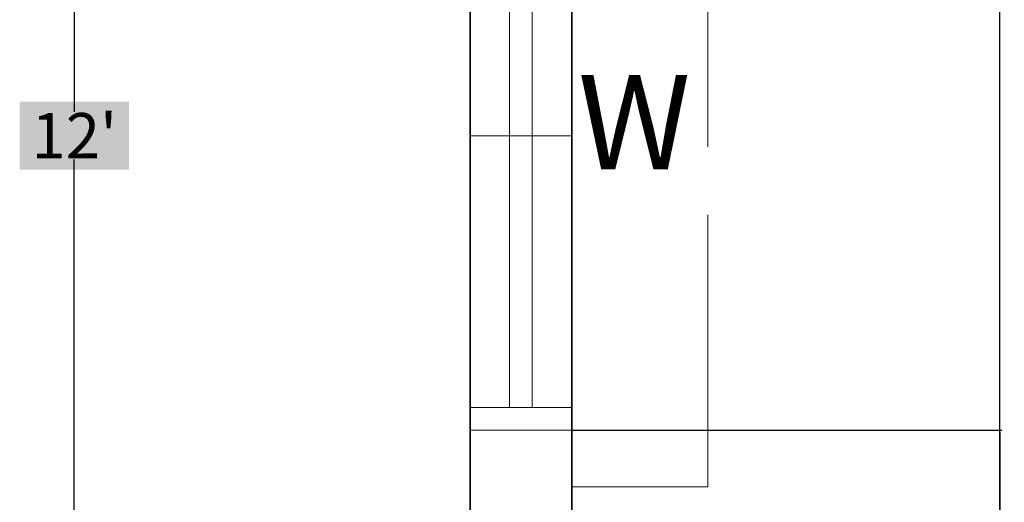
# Model space of a CAD drawing. Units: inches. Extents: x -128 to 854, y -395 to 398.
# Tile 29 of 61: x 265 to 352, y -41 to 2. Entities that reach past the tile are written whole.
import ezdxf

# ---------------------------------------------------------------- set-up
doc = ezdxf.new("R2010")
doc.units = ezdxf.units.IN
doc.header["$MEASUREMENT"] = 0
doc.linetypes.add('ACAD_ISO02W100', pattern=[15, 12, -3])
for name, color, linetype, lineweight in [('A-ANNO-DIMS', 2, 'Continuous', 18), ('A-ANNO-TEXT', 2, 'Continuous', 18), ('A-GLAZ', 220, 'Continuous', 18), ('A-GLAZ-OVHD', 220, 'ACAD_ISO02W100', 13), ('A-WALL', 4, 'Continuous', 35)]:
    doc.layers.add(name, color=color, linetype=linetype, lineweight=lineweight)
doc.styles.get("Standard").update_dxf_attribs({"font": 'arial.ttf'})
doc.dimstyles.get("Standard").update_dxf_attribs({"dimtxt": 0.18, "dimasz": 0.18, "dimexe": 0.18, "dimexo": 0.0625, "dimgap": 0.09, "dimtad": 0, "dimtih": 1, "dimtoh": 1, "dimdec": 1, "dimzin": 0, "dimdsep": 46, "dimlunit": 4, "dimtxsty": 'Standard', "dimcen": 0.09, "dimclrd": 1, "dimclre": 2, "dimclrt": 6, "dimadec": 0, "dimazin": 0, "dimtfac": 1, "dimtdec": 1, "dimtofl": 0, "dimtmove": 0, "dimatfit": 3, "dimfxl": 1, "dimtfill": 2, "dimtfillclr": 3, "dimtolj": 1, "dimtzin": 0, "dimarcsym": 0})

# ---------------------------------------------------------------- blocks, each defined once
blk = doc.blocks.new('*D42')
at = {"layer": 'A-ANNO-DIMS', "color": 0, "lineweight": -2, "transparency": 16777216}
for p, q in [((304.81, 63.741), (269.747, 63.741)), ((269.927, 58.741), (269.927, -6.161)), ((269.927, -75.259), (269.927, -10.358)), ((304.81, -80.259), (269.747, -80.259))]:
    blk.add_line(p, q, dxfattribs=at)
at = {"layer": 'A-ANNO-DIMS', "color": 0, "transparency": 16777216}
for points in [[(269.093, 58.741), (270.76, 58.741), (269.927, 63.741)], [(269.093, -75.259), (270.76, -75.259), (269.927, -80.259)]]:
    blk.add_solid(points, dxfattribs=at)
at = {"layer": 'Defpoints', "color": 0, "transparency": 16777216}
for p in [(269.927, 63.741), (304.873, 63.741), (304.873, -80.259)]:
    blk.add_point(p, dxfattribs=at)
at = {"layer": 'A-ANNO-DIMS', "color": 0, "transparency": 16777216, "insert": (269.927, -8.259), "char_height": 4, "attachment_point": 5, "bg_fill": 1, "box_fill_scale": 1.25, "bg_fill_color": 3, "bg_fill_transparency": 0}
blk.add_mtext("\\A1;12'", dxfattribs=at)
blk = doc.blocks.new('WIN-48IN')
for p, q in [((9, 52), (0, 52)), ((9, 50), (0, 50)), ((3.5, 50), (3.5, 2)), ((5.5, 50), (5.5, 2)), ((9, 26), (0, 26)), ((9, 2), (0, 2)), ((9, 0), (0, 0))]:
    blk.add_line(p, q)
blk = doc.blocks.new('SHADE-48IN')
at = {"ltscale": 2}
for p, q in [((12, 62), (0, 62)), ((0, 0), (0, 62)), ((12, 57), (12, 62)), ((12, 5), (12, 0)), ((12, 0), (0, 0))]:
    blk.add_line(p, q, dxfattribs=at)
blk = doc.blocks.new('*D98')
at = {"layer": 'A-ANNO-DIMS', "color": 2, "lineweight": -2, "transparency": 16777216}
for p, q in [((313.935, 348.741), (351.853, 348.741)), ((313.935, -89.259), (351.853, -89.259))]:
    blk.add_line(p, q, dxfattribs=at)
at = {"layer": 'A-ANNO-DIMS', "color": 1, "lineweight": -2, "transparency": 16777216}
for p, q in [((351.673, 348.561), (351.673, 129.923)), ((351.673, -89.079), (351.673, 129.559))]:
    blk.add_line(p, q, dxfattribs=at)
at = {"layer": 'A-ANNO-DIMS', "color": 1, "transparency": 16777216}
for points in [[(351.643, 348.561), (351.703, 348.561), (351.673, 348.741)], [(351.643, -89.079), (351.703, -89.079), (351.673, -89.259)]]:
    blk.add_solid(points, dxfattribs=at)
at = {"layer": 'Defpoints', "color": 0, "transparency": 16777216}
for p in [(313.873, 348.741), (351.673, 348.741), (313.873, -89.259)]:
    blk.add_point(p, dxfattribs=at)
at = {"layer": 'A-ANNO-DIMS', "color": 6, "transparency": 16777216, "insert": (351.673, 129.741), "char_height": 0.18, "attachment_point": 5, "bg_fill": 1, "box_fill_scale": 1.25, "bg_fill_color": 3, "bg_fill_transparency": 0}
blk.add_mtext('\\A1;36\'-6"', dxfattribs=at)
blk = doc.blocks.new('*D111')
at = {"layer": 'A-ANNO-DIMS', "color": 2, "lineweight": -2, "transparency": 16777216}
for p, q in [((313.935196, -34.259459), (351.852696, -34.259459)), ((313.935196, -89.259459), (351.852696, -89.259459))]:
    blk.add_line(p, q, dxfattribs=at)
at = {"layer": 'A-ANNO-DIMS', "color": 1, "lineweight": -2, "transparency": 16777216}
for p, q in [((351.672696, -34.439459), (351.672696, -61.579459)), ((351.672696, -89.079459), (351.672696, -61.939459))]:
    blk.add_line(p, q, dxfattribs=at)
at = {"layer": 'A-ANNO-DIMS', "color": 1, "transparency": 16777216}
for points in [[(351.642696, -34.439459), (351.702696, -34.439459), (351.672696, -34.259459)], [(351.642696, -89.079459), (351.702696, -89.079459), (351.672696, -89.259459)]]:
    blk.add_solid(points, dxfattribs=at)
at = {"layer": 'Defpoints', "color": 0, "transparency": 16777216}
for p in [(313.872696, -34.259459), (351.672696, -34.259459), (313.872696, -89.259459)]:
    blk.add_point(p, dxfattribs=at)
at = {"layer": 'A-ANNO-DIMS', "color": 6, "transparency": 16777216, "insert": (351.672696, -61.759459), "char_height": 0.18, "attachment_point": 5, "bg_fill": 1, "box_fill_scale": 1.25, "bg_fill_color": 3, "bg_fill_transparency": 0}
blk.add_mtext('\\A1;4\'-7"', dxfattribs=at)

msp = doc.modelspace()

# ---------------------------------------------------------------- linework, layer by layer
at = {"layer": 'A-WALL'}
for p, q in [((313.873, 348.741), (313.873, -89.259)), ((304.873, 63.741), (304.873, -80.259))]:
    msp.add_line(p, q, dxfattribs=at)

# ---------------------------------------------------------------- block references
at = {"layer": 'A-GLAZ', "rotation": 180}
msp.add_blockref('WIN-48IN', (313.873, 17.741), dxfattribs=at)
at = {"layer": 'A-GLAZ-OVHD', "extrusion": (0, 0, -1), "zscale": -1}
msp.add_blockref('SHADE-48IN', (-325.873, -39.259), dxfattribs=at)

# ---------------------------------------------------------------- texts
at = {"layer": 'A-ANNO-TEXT'}
msp.add_text('W', height=8.314, dxfattribs=at).set_placement((314.404, -11.228))

# ---------------------------------------------------------------- dimensions: what is measured, and where the dimension line sits
at = {"layer": 'A-ANNO-DIMS'}
for base, p1, p2, override, picture, middle in [((351.673, 348.741), (313.873, -89.259), (313.873, 348.741), {"dimdec": 1, "dimlfac": 1, "dimrnd": 0, "dimzin": 1, "dimdsep": 46, "dimlunit": 4, "dimfrac": 2}, '*D98', (351.673, 129.741)), ((269.927, 63.741), (304.873, -80.259), (304.873, 63.741), {"dimtxt": 4, "dimasz": 5, "dimclrd": 0, "dimclre": 0, "dimclrt": 0}, '*D42', (269.927, -8.259)), ((351.673, -34.259), (313.873, -89.259), (313.873, -34.259), {"dimdec": 1, "dimlfac": 1, "dimrnd": 0, "dimzin": 1, "dimdsep": 46, "dimlunit": 4, "dimfrac": 2}, '*D111', (351.673, -61.759))]:
    dim = msp.add_linear_dim(base=base, p1=p1, p2=p2, angle=90, dimstyle='Standard', override=override, dxfattribs=at)
    dim.commit()
    dim.dimension.update_dxf_attribs({"geometry": picture, "text_midpoint": middle})

doc.saveas('drawing.dxf')
